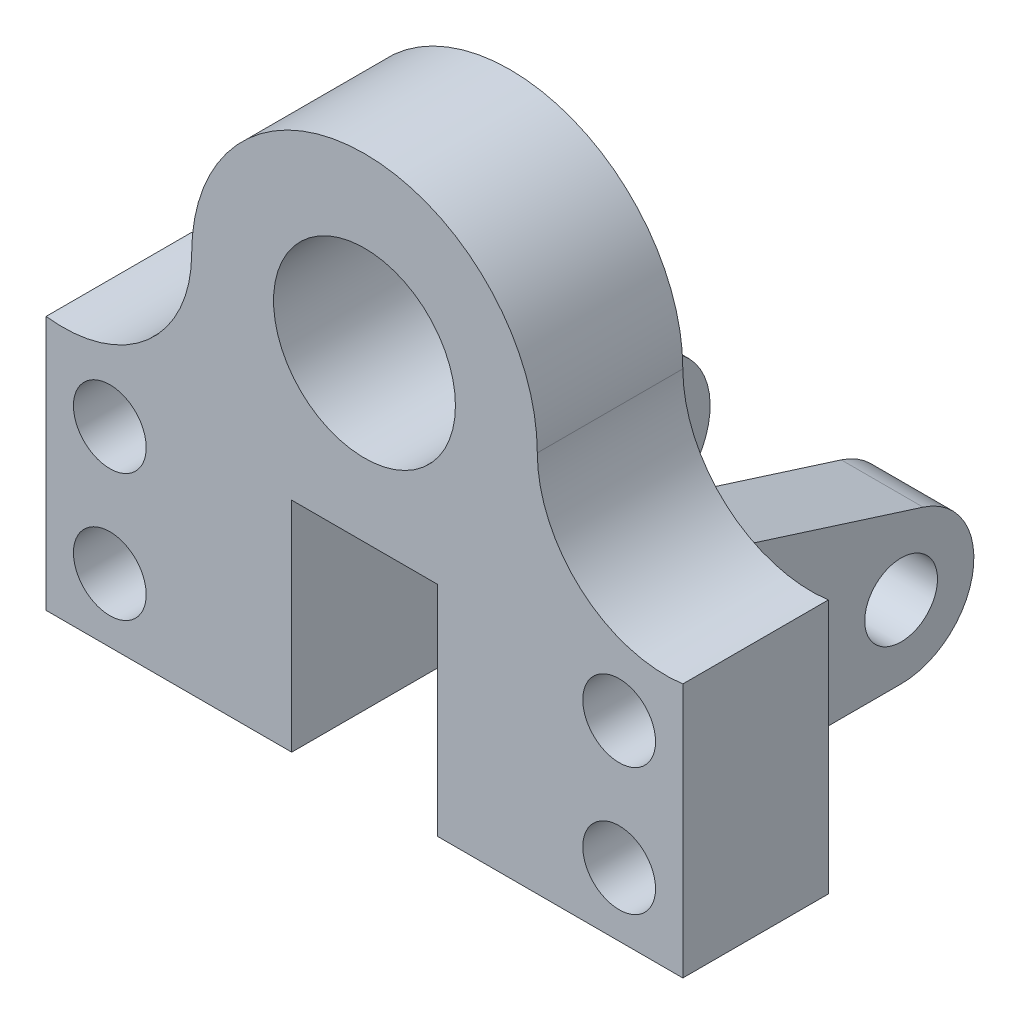
ISO-10303-21;
HEADER;
FILE_DESCRIPTION(('STEP AP214'),'2;1');
FILE_NAME('part.step','',(''),(''),'','','');
FILE_SCHEMA(('AUTOMOTIVE_DESIGN { 1 0 10303 214 1 1 1 1 }'));
ENDSEC;
DATA;
#1=APPLICATION_CONTEXT('core data for automotive mechanical design processes');
#2=APPLICATION_PROTOCOL_DEFINITION('international standard','automotive_design',2000,#1);
#3=PRODUCT_CONTEXT('',#1,'mechanical');
#4=PRODUCT('Part','Part','',(#3));
#5=PRODUCT_RELATED_PRODUCT_CATEGORY('part','',(#4));
#6=PRODUCT_DEFINITION_FORMATION('','',#4);
#7=PRODUCT_DEFINITION_CONTEXT('part definition',#1,'design');
#8=PRODUCT_DEFINITION('design','',#6,#7);
#9=PRODUCT_DEFINITION_SHAPE('','',#8);
#10=(LENGTH_UNIT() NAMED_UNIT(*) SI_UNIT(.MILLI.,.METRE.));
#11=(NAMED_UNIT(*) PLANE_ANGLE_UNIT() SI_UNIT($,.RADIAN.));
#12=(NAMED_UNIT(*) SI_UNIT($,.STERADIAN.) SOLID_ANGLE_UNIT());
#13=UNCERTAINTY_MEASURE_WITH_UNIT(LENGTH_MEASURE(1.E-05),#10,'distance_accuracy_value','');
#14=(GEOMETRIC_REPRESENTATION_CONTEXT(3) GLOBAL_UNCERTAINTY_ASSIGNED_CONTEXT((#13)) GLOBAL_UNIT_ASSIGNED_CONTEXT((#10,
#11,#12)) REPRESENTATION_CONTEXT('',''));
#15=CARTESIAN_POINT('',(0.,0.,0.));
#16=DIRECTION('',(0.,0.,1.));
#17=DIRECTION('',(1.,0.,0.));
#18=AXIS2_PLACEMENT_3D('',#15,#16,#17);
#19=CARTESIAN_POINT('',(-66.25,36.,-16.));
#20=DIRECTION('',(0.,0.,-1.));
#21=DIRECTION('',(-1.,0.,0.));
#22=AXIS2_PLACEMENT_3D('',#19,#20,#21);
#23=PLANE('',#22);
#24=DIRECTION('',(0.,-1.,0.));
#25=VECTOR('',#24,1.);
#26=CARTESIAN_POINT('',(-38.,0.,-16.));
#27=LINE('',#26,#25);
#28=CARTESIAN_POINT('',(-38.,0.,-16.));
#29=VERTEX_POINT('',#28);
#30=CARTESIAN_POINT('',(-38.,-48.,-16.));
#31=VERTEX_POINT('',#30);
#32=EDGE_CURVE('E164',#29,#31,#27,.T.);
#33=ORIENTED_EDGE('',*,*,#32,.T.);
#34=DIRECTION('',(1.,0.,0.));
#35=VECTOR('',#34,1.);
#36=CARTESIAN_POINT('',(-16.,-48.,-16.));
#37=LINE('',#36,#35);
#38=CARTESIAN_POINT('',(-70.,-48.,-16.));
#39=VERTEX_POINT('',#38);
#40=EDGE_CURVE('E283',#39,#31,#37,.T.);
#41=ORIENTED_EDGE('',*,*,#40,.F.);
#42=DIRECTION('',(0.,-1.,0.));
#43=VECTOR('',#42,1.);
#44=CARTESIAN_POINT('',(-70.,-48.,-16.));
#45=LINE('',#44,#43);
#46=CARTESIAN_POINT('',(-70.,8.,-16.));
#47=VERTEX_POINT('',#46);
#48=EDGE_CURVE('E285',#47,#39,#45,.T.);
#49=ORIENTED_EDGE('',*,*,#48,.F.);
#50=CARTESIAN_POINT('',(-66.25,36.,-16.));
#51=DIRECTION('',(0.,0.,-1.));
#52=DIRECTION('',(-1.,0.,0.));
#53=AXIS2_PLACEMENT_3D('',#50,#51,#52);
#54=CIRCLE('',#53,28.25);
#55=CARTESIAN_POINT('',(-38.,36.,-16.));
#56=VERTEX_POINT('',#55);
#57=EDGE_CURVE('E255',#56,#47,#54,.T.);
#58=ORIENTED_EDGE('',*,*,#57,.F.);
#59=CARTESIAN_POINT('',(0.,36.,-16.));
#60=DIRECTION('',(0.,0.,1.));
#61=DIRECTION('',(1.,0.,0.));
#62=AXIS2_PLACEMENT_3D('',#59,#60,#61);
#63=CIRCLE('',#62,38.);
#64=CARTESIAN_POINT('',(38.,36.,-16.));
#65=VERTEX_POINT('',#64);
#66=EDGE_CURVE('E261',#65,#56,#63,.T.);
#67=ORIENTED_EDGE('',*,*,#66,.F.);
#68=CARTESIAN_POINT('',(66.25,36.,-16.));
#69=DIRECTION('',(0.,0.,-1.));
#70=DIRECTION('',(1.,0.,0.));
#71=AXIS2_PLACEMENT_3D('',#68,#69,#70);
#72=CIRCLE('',#71,28.25);
#73=CARTESIAN_POINT('',(70.,8.,-16.));
#74=VERTEX_POINT('',#73);
#75=EDGE_CURVE('E296',#74,#65,#72,.T.);
#76=ORIENTED_EDGE('',*,*,#75,.F.);
#77=DIRECTION('',(0.,1.,0.));
#78=VECTOR('',#77,1.);
#79=CARTESIAN_POINT('',(70.,-48.,-16.));
#80=LINE('',#79,#78);
#81=CARTESIAN_POINT('',(70.,-48.,-16.));
#82=VERTEX_POINT('',#81);
#83=EDGE_CURVE('E300',#82,#74,#80,.T.);
#84=ORIENTED_EDGE('',*,*,#83,.F.);
#85=DIRECTION('',(1.,0.,0.));
#86=VECTOR('',#85,1.);
#87=CARTESIAN_POINT('',(16.,-48.,-16.));
#88=LINE('',#87,#86);
#89=CARTESIAN_POINT('',(38.,-48.,-16.));
#90=VERTEX_POINT('',#89);
#91=EDGE_CURVE('E291',#90,#82,#88,.T.);
#92=ORIENTED_EDGE('',*,*,#91,.F.);
#93=DIRECTION('',(0.,-1.,0.));
#94=VECTOR('',#93,1.);
#95=CARTESIAN_POINT('',(38.,0.,-16.));
#96=LINE('',#95,#94);
#97=CARTESIAN_POINT('',(38.,0.,-16.));
#98=VERTEX_POINT('',#97);
#99=EDGE_CURVE('E203',#98,#90,#96,.T.);
#100=ORIENTED_EDGE('',*,*,#99,.F.);
#101=DIRECTION('',(-1.,0.,0.));
#102=VECTOR('',#101,1.);
#103=CARTESIAN_POINT('',(38.,0.,-16.));
#104=LINE('',#103,#102);
#105=CARTESIAN_POINT('',(20.,0.,-16.));
#106=VERTEX_POINT('',#105);
#107=EDGE_CURVE('E211',#98,#106,#104,.T.);
#108=ORIENTED_EDGE('',*,*,#107,.T.);
#109=DIRECTION('',(0.,-1.,0.));
#110=VECTOR('',#109,1.);
#111=CARTESIAN_POINT('',(20.,0.,-16.));
#112=LINE('',#111,#110);
#113=CARTESIAN_POINT('',(20.,-48.,-16.));
#114=VERTEX_POINT('',#113);
#115=EDGE_CURVE('E65',#106,#114,#112,.T.);
#116=ORIENTED_EDGE('',*,*,#115,.T.);
#117=CARTESIAN_POINT('',(16.,-48.,-16.));
#118=VERTEX_POINT('',#117);
#119=EDGE_CURVE('E294',#118,#114,#88,.T.);
#120=ORIENTED_EDGE('',*,*,#119,.F.);
#121=DIRECTION('',(0.,-1.,0.));
#122=VECTOR('',#121,1.);
#123=CARTESIAN_POINT('',(16.,0.,-16.));
#124=LINE('',#123,#122);
#125=CARTESIAN_POINT('',(16.,0.,-16.));
#126=VERTEX_POINT('',#125);
#127=EDGE_CURVE('E292',#126,#118,#124,.T.);
#128=ORIENTED_EDGE('',*,*,#127,.F.);
#129=DIRECTION('',(1.,0.,0.));
#130=VECTOR('',#129,1.);
#131=CARTESIAN_POINT('',(-16.,0.,-16.));
#132=LINE('',#131,#130);
#133=CARTESIAN_POINT('',(-16.,0.,-16.));
#134=VERTEX_POINT('',#133);
#135=EDGE_CURVE('E287',#134,#126,#132,.T.);
#136=ORIENTED_EDGE('',*,*,#135,.F.);
#137=DIRECTION('',(0.,1.,0.));
#138=VECTOR('',#137,1.);
#139=CARTESIAN_POINT('',(-16.,0.,-16.));
#140=LINE('',#139,#138);
#141=CARTESIAN_POINT('',(-16.,-48.,-16.));
#142=VERTEX_POINT('',#141);
#143=EDGE_CURVE('E290',#142,#134,#140,.T.);
#144=ORIENTED_EDGE('',*,*,#143,.F.);
#145=CARTESIAN_POINT('',(-20.,-48.,-16.));
#146=VERTEX_POINT('',#145);
#147=EDGE_CURVE('E281',#146,#142,#37,.T.);
#148=ORIENTED_EDGE('',*,*,#147,.F.);
#149=DIRECTION('',(0.,-1.,0.));
#150=VECTOR('',#149,1.);
#151=CARTESIAN_POINT('',(-20.,0.,-16.));
#152=LINE('',#151,#150);
#153=CARTESIAN_POINT('',(-20.,0.,-16.));
#154=VERTEX_POINT('',#153);
#155=EDGE_CURVE('E186',#154,#146,#152,.T.);
#156=ORIENTED_EDGE('',*,*,#155,.F.);
#157=DIRECTION('',(1.,0.,0.));
#158=VECTOR('',#157,1.);
#159=CARTESIAN_POINT('',(-38.,0.,-16.));
#160=LINE('',#159,#158);
#161=EDGE_CURVE('E182',#29,#154,#160,.T.);
#162=ORIENTED_EDGE('',*,*,#161,.F.);
#163=EDGE_LOOP('',(#33,#41,#49,#58,#67,#76,#84,#92,#100,#108,#116,#120,#128,#136,#144,#148,#156,#162));
#164=FACE_BOUND('',#163,.T.);
#165=CARTESIAN_POINT('',(-56.,-34.,-16.));
#166=DIRECTION('',(0.,0.,1.));
#167=DIRECTION('',(-1.,0.,0.));
#168=AXIS2_PLACEMENT_3D('',#165,#166,#167);
#169=CIRCLE('',#168,8.00000000000001);
#170=CARTESIAN_POINT('',(-64.,-34.,-16.));
#171=VERTEX_POINT('',#170);
#172=EDGE_CURVE('E228',#171,#171,#169,.T.);
#173=ORIENTED_EDGE('',*,*,#172,.T.);
#174=EDGE_LOOP('',(#173));
#175=FACE_BOUND('',#174,.T.);
#176=CARTESIAN_POINT('',(56.,-34.,-16.));
#177=DIRECTION('',(0.,0.,1.));
#178=DIRECTION('',(1.,0.,0.));
#179=AXIS2_PLACEMENT_3D('',#176,#177,#178);
#180=CIRCLE('',#179,8.00000000000001);
#181=CARTESIAN_POINT('',(64.,-34.,-16.));
#182=VERTEX_POINT('',#181);
#183=EDGE_CURVE('E245',#182,#182,#180,.T.);
#184=ORIENTED_EDGE('',*,*,#183,.T.);
#185=EDGE_LOOP('',(#184));
#186=FACE_BOUND('',#185,.T.);
#187=CARTESIAN_POINT('',(0.,36.,-16.));
#188=DIRECTION('',(0.,0.,1.));
#189=DIRECTION('',(1.,0.,0.));
#190=AXIS2_PLACEMENT_3D('',#187,#188,#189);
#191=CIRCLE('',#190,20.);
#192=CARTESIAN_POINT('',(20.,36.,-16.));
#193=VERTEX_POINT('',#192);
#194=EDGE_CURVE('E246',#193,#193,#191,.T.);
#195=ORIENTED_EDGE('',*,*,#194,.T.);
#196=EDGE_LOOP('',(#195));
#197=FACE_BOUND('',#196,.T.);
#198=CARTESIAN_POINT('',(56.,-6.,-16.));
#199=DIRECTION('',(0.,0.,1.));
#200=DIRECTION('',(1.,0.,0.));
#201=AXIS2_PLACEMENT_3D('',#198,#199,#200);
#202=CIRCLE('',#201,8.);
#203=CARTESIAN_POINT('',(64.,-6.,-16.));
#204=VERTEX_POINT('',#203);
#205=EDGE_CURVE('E237',#204,#204,#202,.T.);
#206=ORIENTED_EDGE('',*,*,#205,.T.);
#207=EDGE_LOOP('',(#206));
#208=FACE_BOUND('',#207,.T.);
#209=CARTESIAN_POINT('',(-56.,-6.00000000000003,-16.));
#210=DIRECTION('',(0.,0.,1.));
#211=DIRECTION('',(-1.,0.,0.));
#212=AXIS2_PLACEMENT_3D('',#209,#210,#211);
#213=CIRCLE('',#212,8.);
#214=CARTESIAN_POINT('',(-64.,-6.00000000000003,-16.));
#215=VERTEX_POINT('',#214);
#216=EDGE_CURVE('E227',#215,#215,#213,.T.);
#217=ORIENTED_EDGE('',*,*,#216,.T.);
#218=EDGE_LOOP('',(#217));
#219=FACE_BOUND('',#218,.T.);
#220=ADVANCED_FACE('F39',(#164,#175,#186,#197,#208,#219),#23,.T.);
#221=CARTESIAN_POINT('',(-66.25,36.,16.));
#222=DIRECTION('',(0.,0.,-1.));
#223=DIRECTION('',(-1.,0.,0.));
#224=AXIS2_PLACEMENT_3D('',#221,#222,#223);
#225=PLANE('',#224);
#226=CARTESIAN_POINT('',(-66.25,36.,16.));
#227=DIRECTION('',(0.,0.,-1.));
#228=DIRECTION('',(-1.,0.,0.));
#229=AXIS2_PLACEMENT_3D('',#226,#227,#228);
#230=CIRCLE('',#229,28.25);
#231=CARTESIAN_POINT('',(-38.,36.,16.));
#232=VERTEX_POINT('',#231);
#233=CARTESIAN_POINT('',(-70.,8.,16.));
#234=VERTEX_POINT('',#233);
#235=EDGE_CURVE('E260',#232,#234,#230,.T.);
#236=ORIENTED_EDGE('',*,*,#235,.T.);
#237=DIRECTION('',(0.,-1.,0.));
#238=VECTOR('',#237,1.);
#239=CARTESIAN_POINT('',(-70.,-48.,16.));
#240=LINE('',#239,#238);
#241=CARTESIAN_POINT('',(-70.,-48.,16.));
#242=VERTEX_POINT('',#241);
#243=EDGE_CURVE('E257',#234,#242,#240,.T.);
#244=ORIENTED_EDGE('',*,*,#243,.T.);
#245=DIRECTION('',(1.,0.,0.));
#246=VECTOR('',#245,1.);
#247=CARTESIAN_POINT('',(-16.,-48.,16.));
#248=LINE('',#247,#246);
#249=CARTESIAN_POINT('',(-16.,-48.,16.));
#250=VERTEX_POINT('',#249);
#251=EDGE_CURVE('E263',#242,#250,#248,.T.);
#252=ORIENTED_EDGE('',*,*,#251,.T.);
#253=DIRECTION('',(0.,1.,0.));
#254=VECTOR('',#253,1.);
#255=CARTESIAN_POINT('',(-16.,0.,16.));
#256=LINE('',#255,#254);
#257=CARTESIAN_POINT('',(-16.,0.,16.));
#258=VERTEX_POINT('',#257);
#259=EDGE_CURVE('E264',#250,#258,#256,.T.);
#260=ORIENTED_EDGE('',*,*,#259,.T.);
#261=DIRECTION('',(1.,0.,0.));
#262=VECTOR('',#261,1.);
#263=CARTESIAN_POINT('',(-16.,0.,16.));
#264=LINE('',#263,#262);
#265=CARTESIAN_POINT('',(16.,0.,16.));
#266=VERTEX_POINT('',#265);
#267=EDGE_CURVE('E270',#258,#266,#264,.T.);
#268=ORIENTED_EDGE('',*,*,#267,.T.);
#269=DIRECTION('',(0.,-1.,0.));
#270=VECTOR('',#269,1.);
#271=CARTESIAN_POINT('',(16.,0.,16.));
#272=LINE('',#271,#270);
#273=CARTESIAN_POINT('',(16.,-48.,16.));
#274=VERTEX_POINT('',#273);
#275=EDGE_CURVE('E267',#266,#274,#272,.T.);
#276=ORIENTED_EDGE('',*,*,#275,.T.);
#277=DIRECTION('',(1.,0.,0.));
#278=VECTOR('',#277,1.);
#279=CARTESIAN_POINT('',(16.,-48.,16.));
#280=LINE('',#279,#278);
#281=CARTESIAN_POINT('',(70.,-48.,16.));
#282=VERTEX_POINT('',#281);
#283=EDGE_CURVE('E271',#274,#282,#280,.T.);
#284=ORIENTED_EDGE('',*,*,#283,.T.);
#285=DIRECTION('',(0.,1.,0.));
#286=VECTOR('',#285,1.);
#287=CARTESIAN_POINT('',(70.,-48.,16.));
#288=LINE('',#287,#286);
#289=CARTESIAN_POINT('',(70.,8.,16.));
#290=VERTEX_POINT('',#289);
#291=EDGE_CURVE('E272',#282,#290,#288,.T.);
#292=ORIENTED_EDGE('',*,*,#291,.T.);
#293=CARTESIAN_POINT('',(66.25,36.,16.));
#294=DIRECTION('',(0.,0.,-1.));
#295=DIRECTION('',(1.,0.,0.));
#296=AXIS2_PLACEMENT_3D('',#293,#294,#295);
#297=CIRCLE('',#296,28.25);
#298=CARTESIAN_POINT('',(38.,36.,16.));
#299=VERTEX_POINT('',#298);
#300=EDGE_CURVE('E274',#290,#299,#297,.T.);
#301=ORIENTED_EDGE('',*,*,#300,.T.);
#302=CARTESIAN_POINT('',(0.,36.,16.));
#303=DIRECTION('',(0.,0.,1.));
#304=DIRECTION('',(1.,0.,0.));
#305=AXIS2_PLACEMENT_3D('',#302,#303,#304);
#306=CIRCLE('',#305,38.);
#307=EDGE_CURVE('E280',#299,#232,#306,.T.);
#308=ORIENTED_EDGE('',*,*,#307,.T.);
#309=EDGE_LOOP('',(#236,#244,#252,#260,#268,#276,#284,#292,#301,#308));
#310=FACE_BOUND('',#309,.T.);
#311=CARTESIAN_POINT('',(0.,36.,16.));
#312=DIRECTION('',(0.,0.,1.));
#313=DIRECTION('',(1.,0.,0.));
#314=AXIS2_PLACEMENT_3D('',#311,#312,#313);
#315=CIRCLE('',#314,20.);
#316=CARTESIAN_POINT('',(20.,36.,16.));
#317=VERTEX_POINT('',#316);
#318=EDGE_CURVE('E253',#317,#317,#315,.T.);
#319=ORIENTED_EDGE('',*,*,#318,.F.);
#320=EDGE_LOOP('',(#319));
#321=FACE_BOUND('',#320,.T.);
#322=CARTESIAN_POINT('',(56.,-34.,16.));
#323=DIRECTION('',(0.,0.,1.));
#324=DIRECTION('',(1.,0.,0.));
#325=AXIS2_PLACEMENT_3D('',#322,#323,#324);
#326=CIRCLE('',#325,8.00000000000001);
#327=CARTESIAN_POINT('',(64.,-34.,16.));
#328=VERTEX_POINT('',#327);
#329=EDGE_CURVE('E243',#328,#328,#326,.T.);
#330=ORIENTED_EDGE('',*,*,#329,.F.);
#331=EDGE_LOOP('',(#330));
#332=FACE_BOUND('',#331,.T.);
#333=CARTESIAN_POINT('',(56.,-6.,16.));
#334=DIRECTION('',(0.,0.,1.));
#335=DIRECTION('',(1.,0.,0.));
#336=AXIS2_PLACEMENT_3D('',#333,#334,#335);
#337=CIRCLE('',#336,8.);
#338=CARTESIAN_POINT('',(64.,-6.,16.));
#339=VERTEX_POINT('',#338);
#340=EDGE_CURVE('E239',#339,#339,#337,.T.);
#341=ORIENTED_EDGE('',*,*,#340,.F.);
#342=EDGE_LOOP('',(#341));
#343=FACE_BOUND('',#342,.T.);
#344=CARTESIAN_POINT('',(-56.,-34.,16.));
#345=DIRECTION('',(0.,0.,1.));
#346=DIRECTION('',(-1.,0.,0.));
#347=AXIS2_PLACEMENT_3D('',#344,#345,#346);
#348=CIRCLE('',#347,8.00000000000001);
#349=CARTESIAN_POINT('',(-64.,-34.,16.));
#350=VERTEX_POINT('',#349);
#351=EDGE_CURVE('E231',#350,#350,#348,.T.);
#352=ORIENTED_EDGE('',*,*,#351,.F.);
#353=EDGE_LOOP('',(#352));
#354=FACE_BOUND('',#353,.T.);
#355=CARTESIAN_POINT('',(-56.,-6.00000000000003,16.));
#356=DIRECTION('',(0.,0.,1.));
#357=DIRECTION('',(-1.,0.,0.));
#358=AXIS2_PLACEMENT_3D('',#355,#356,#357);
#359=CIRCLE('',#358,8.);
#360=CARTESIAN_POINT('',(-64.,-6.00000000000003,16.));
#361=VERTEX_POINT('',#360);
#362=EDGE_CURVE('E230',#361,#361,#359,.T.);
#363=ORIENTED_EDGE('',*,*,#362,.F.);
#364=EDGE_LOOP('',(#363));
#365=FACE_BOUND('',#364,.T.);
#366=ADVANCED_FACE('F389',(#310,#321,#332,#343,#354,#365),#225,.F.);
#367=CARTESIAN_POINT('',(-66.25,36.,16.));
#368=DIRECTION('',(0.,0.,-1.));
#369=DIRECTION('',(-1.,0.,0.));
#370=AXIS2_PLACEMENT_3D('',#367,#368,#369);
#371=CYLINDRICAL_SURFACE('',#370,28.25);
#372=ORIENTED_EDGE('',*,*,#57,.T.);
#373=DIRECTION('',(0.,0.,-1.));
#374=VECTOR('',#373,1.);
#375=CARTESIAN_POINT('',(-70.,8.,16.));
#376=LINE('',#375,#374);
#377=EDGE_CURVE('E11',#234,#47,#376,.T.);
#378=ORIENTED_EDGE('',*,*,#377,.F.);
#379=ORIENTED_EDGE('',*,*,#235,.F.);
#380=DIRECTION('',(0.,0.,-1.));
#381=VECTOR('',#380,1.);
#382=CARTESIAN_POINT('',(-38.,36.,16.));
#383=LINE('',#382,#381);
#384=EDGE_CURVE('E276',#232,#56,#383,.T.);
#385=ORIENTED_EDGE('',*,*,#384,.T.);
#386=EDGE_LOOP('',(#372,#378,#379,#385));
#387=FACE_BOUND('',#386,.T.);
#388=ADVANCED_FACE('F41',(#387),#371,.F.);
#389=CARTESIAN_POINT('',(-70.,-48.,16.));
#390=DIRECTION('',(1.,0.,0.));
#391=DIRECTION('',(0.,0.,-1.));
#392=AXIS2_PLACEMENT_3D('',#389,#390,#391);
#393=PLANE('',#392);
#394=ORIENTED_EDGE('',*,*,#48,.T.);
#395=DIRECTION('',(0.,0.,-1.));
#396=VECTOR('',#395,1.);
#397=CARTESIAN_POINT('',(-70.,-48.,16.));
#398=LINE('',#397,#396);
#399=EDGE_CURVE('E50',#242,#39,#398,.T.);
#400=ORIENTED_EDGE('',*,*,#399,.F.);
#401=ORIENTED_EDGE('',*,*,#243,.F.);
#402=ORIENTED_EDGE('',*,*,#377,.T.);
#403=EDGE_LOOP('',(#394,#400,#401,#402));
#404=FACE_BOUND('',#403,.T.);
#405=ADVANCED_FACE('F334',(#404),#393,.F.);
#406=CARTESIAN_POINT('',(-16.,-48.,16.));
#407=DIRECTION('',(0.,1.,0.));
#408=DIRECTION('',(0.,0.,1.));
#409=AXIS2_PLACEMENT_3D('',#406,#407,#408);
#410=PLANE('',#409);
#411=ORIENTED_EDGE('',*,*,#40,.T.);
#412=DIRECTION('',(0.,0.,-1.));
#413=VECTOR('',#412,1.);
#414=CARTESIAN_POINT('',(-38.,-48.,-16.));
#415=LINE('',#414,#413);
#416=CARTESIAN_POINT('',(-38.,-48.,-64.));
#417=VERTEX_POINT('',#416);
#418=EDGE_CURVE('E175',#31,#417,#415,.T.);
#419=ORIENTED_EDGE('',*,*,#418,.T.);
#420=DIRECTION('',(1.,0.,0.));
#421=VECTOR('',#420,1.);
#422=CARTESIAN_POINT('',(-38.,-48.,-64.));
#423=LINE('',#422,#421);
#424=CARTESIAN_POINT('',(-20.,-48.,-64.));
#425=VERTEX_POINT('',#424);
#426=EDGE_CURVE('E194',#417,#425,#423,.T.);
#427=ORIENTED_EDGE('',*,*,#426,.T.);
#428=DIRECTION('',(0.,0.,-1.));
#429=VECTOR('',#428,1.);
#430=CARTESIAN_POINT('',(-20.,-48.,-16.));
#431=LINE('',#430,#429);
#432=EDGE_CURVE('E53',#146,#425,#431,.T.);
#433=ORIENTED_EDGE('',*,*,#432,.F.);
#434=ORIENTED_EDGE('',*,*,#147,.T.);
#435=DIRECTION('',(0.,0.,-1.));
#436=VECTOR('',#435,1.);
#437=CARTESIAN_POINT('',(-16.,-48.,16.));
#438=LINE('',#437,#436);
#439=EDGE_CURVE('E325',#250,#142,#438,.T.);
#440=ORIENTED_EDGE('',*,*,#439,.F.);
#441=ORIENTED_EDGE('',*,*,#251,.F.);
#442=ORIENTED_EDGE('',*,*,#399,.T.);
#443=EDGE_LOOP('',(#411,#419,#427,#433,#434,#440,#441,#442));
#444=FACE_BOUND('',#443,.T.);
#445=ADVANCED_FACE('F330',(#444),#410,.F.);
#446=CARTESIAN_POINT('',(-16.,0.,16.));
#447=DIRECTION('',(-1.,0.,0.));
#448=DIRECTION('',(0.,-1.,0.));
#449=AXIS2_PLACEMENT_3D('',#446,#447,#448);
#450=PLANE('',#449);
#451=ORIENTED_EDGE('',*,*,#143,.T.);
#452=DIRECTION('',(0.,0.,-1.));
#453=VECTOR('',#452,1.);
#454=CARTESIAN_POINT('',(-16.,0.,16.));
#455=LINE('',#454,#453);
#456=EDGE_CURVE('E317',#258,#134,#455,.T.);
#457=ORIENTED_EDGE('',*,*,#456,.F.);
#458=ORIENTED_EDGE('',*,*,#259,.F.);
#459=ORIENTED_EDGE('',*,*,#439,.T.);
#460=EDGE_LOOP('',(#451,#457,#458,#459));
#461=FACE_BOUND('',#460,.T.);
#462=ADVANCED_FACE('F387',(#461),#450,.F.);
#463=CARTESIAN_POINT('',(-16.,0.,16.));
#464=DIRECTION('',(0.,1.,0.));
#465=DIRECTION('',(0.,0.,1.));
#466=AXIS2_PLACEMENT_3D('',#463,#464,#465);
#467=PLANE('',#466);
#468=ORIENTED_EDGE('',*,*,#135,.T.);
#469=DIRECTION('',(0.,0.,-1.));
#470=VECTOR('',#469,1.);
#471=CARTESIAN_POINT('',(16.,0.,16.));
#472=LINE('',#471,#470);
#473=EDGE_CURVE('E316',#266,#126,#472,.T.);
#474=ORIENTED_EDGE('',*,*,#473,.F.);
#475=ORIENTED_EDGE('',*,*,#267,.F.);
#476=ORIENTED_EDGE('',*,*,#456,.T.);
#477=EDGE_LOOP('',(#468,#474,#475,#476));
#478=FACE_BOUND('',#477,.T.);
#479=ADVANCED_FACE('F385',(#478),#467,.F.);
#480=CARTESIAN_POINT('',(16.,0.,16.));
#481=DIRECTION('',(1.,0.,0.));
#482=DIRECTION('',(0.,1.,0.));
#483=AXIS2_PLACEMENT_3D('',#480,#481,#482);
#484=PLANE('',#483);
#485=ORIENTED_EDGE('',*,*,#127,.T.);
#486=DIRECTION('',(0.,0.,-1.));
#487=VECTOR('',#486,1.);
#488=CARTESIAN_POINT('',(16.,-48.,16.));
#489=LINE('',#488,#487);
#490=EDGE_CURVE('E311',#274,#118,#489,.T.);
#491=ORIENTED_EDGE('',*,*,#490,.F.);
#492=ORIENTED_EDGE('',*,*,#275,.F.);
#493=ORIENTED_EDGE('',*,*,#473,.T.);
#494=EDGE_LOOP('',(#485,#491,#492,#493));
#495=FACE_BOUND('',#494,.T.);
#496=ADVANCED_FACE('F380',(#495),#484,.F.);
#497=CARTESIAN_POINT('',(16.,-48.,16.));
#498=DIRECTION('',(0.,1.,0.));
#499=DIRECTION('',(0.,0.,1.));
#500=AXIS2_PLACEMENT_3D('',#497,#498,#499);
#501=PLANE('',#500);
#502=ORIENTED_EDGE('',*,*,#119,.T.);
#503=DIRECTION('',(0.,0.,-1.));
#504=VECTOR('',#503,1.);
#505=CARTESIAN_POINT('',(20.,-48.,-16.));
#506=LINE('',#505,#504);
#507=CARTESIAN_POINT('',(20.,-48.,-64.));
#508=VERTEX_POINT('',#507);
#509=EDGE_CURVE('E213',#114,#508,#506,.T.);
#510=ORIENTED_EDGE('',*,*,#509,.T.);
#511=DIRECTION('',(-1.,0.,0.));
#512=VECTOR('',#511,1.);
#513=CARTESIAN_POINT('',(38.,-48.,-64.));
#514=LINE('',#513,#512);
#515=CARTESIAN_POINT('',(38.,-48.,-64.));
#516=VERTEX_POINT('',#515);
#517=EDGE_CURVE('E224',#516,#508,#514,.T.);
#518=ORIENTED_EDGE('',*,*,#517,.F.);
#519=DIRECTION('',(0.,0.,-1.));
#520=VECTOR('',#519,1.);
#521=CARTESIAN_POINT('',(38.,-48.,-16.));
#522=LINE('',#521,#520);
#523=EDGE_CURVE('E204',#90,#516,#522,.T.);
#524=ORIENTED_EDGE('',*,*,#523,.F.);
#525=ORIENTED_EDGE('',*,*,#91,.T.);
#526=DIRECTION('',(0.,0.,-1.));
#527=VECTOR('',#526,1.);
#528=CARTESIAN_POINT('',(70.,-48.,16.));
#529=LINE('',#528,#527);
#530=EDGE_CURVE('E309',#282,#82,#529,.T.);
#531=ORIENTED_EDGE('',*,*,#530,.F.);
#532=ORIENTED_EDGE('',*,*,#283,.F.);
#533=ORIENTED_EDGE('',*,*,#490,.T.);
#534=EDGE_LOOP('',(#502,#510,#518,#524,#525,#531,#532,#533));
#535=FACE_BOUND('',#534,.T.);
#536=ADVANCED_FACE('F351',(#535),#501,.F.);
#537=CARTESIAN_POINT('',(70.,-48.,16.));
#538=DIRECTION('',(-1.,0.,0.));
#539=DIRECTION('',(0.,0.,1.));
#540=AXIS2_PLACEMENT_3D('',#537,#538,#539);
#541=PLANE('',#540);
#542=ORIENTED_EDGE('',*,*,#83,.T.);
#543=DIRECTION('',(0.,0.,-1.));
#544=VECTOR('',#543,1.);
#545=CARTESIAN_POINT('',(70.,8.,16.));
#546=LINE('',#545,#544);
#547=EDGE_CURVE('E307',#290,#74,#546,.T.);
#548=ORIENTED_EDGE('',*,*,#547,.F.);
#549=ORIENTED_EDGE('',*,*,#291,.F.);
#550=ORIENTED_EDGE('',*,*,#530,.T.);
#551=EDGE_LOOP('',(#542,#548,#549,#550));
#552=FACE_BOUND('',#551,.T.);
#553=ADVANCED_FACE('F348',(#552),#541,.F.);
#554=CARTESIAN_POINT('',(66.25,36.,16.));
#555=DIRECTION('',(0.,0.,-1.));
#556=DIRECTION('',(-1.,0.,0.));
#557=AXIS2_PLACEMENT_3D('',#554,#555,#556);
#558=CYLINDRICAL_SURFACE('',#557,28.25);
#559=ORIENTED_EDGE('',*,*,#75,.T.);
#560=DIRECTION('',(0.,0.,-1.));
#561=VECTOR('',#560,1.);
#562=CARTESIAN_POINT('',(38.,36.,16.));
#563=LINE('',#562,#561);
#564=EDGE_CURVE('E302',#299,#65,#563,.T.);
#565=ORIENTED_EDGE('',*,*,#564,.F.);
#566=ORIENTED_EDGE('',*,*,#300,.F.);
#567=ORIENTED_EDGE('',*,*,#547,.T.);
#568=EDGE_LOOP('',(#559,#565,#566,#567));
#569=FACE_BOUND('',#568,.T.);
#570=ADVANCED_FACE('F344',(#569),#558,.F.);
#571=CARTESIAN_POINT('',(0.,36.,16.));
#572=DIRECTION('',(0.,0.,-1.));
#573=DIRECTION('',(-1.,0.,0.));
#574=AXIS2_PLACEMENT_3D('',#571,#572,#573);
#575=CYLINDRICAL_SURFACE('',#574,38.);
#576=ORIENTED_EDGE('',*,*,#66,.T.);
#577=ORIENTED_EDGE('',*,*,#384,.F.);
#578=ORIENTED_EDGE('',*,*,#307,.F.);
#579=ORIENTED_EDGE('',*,*,#564,.T.);
#580=EDGE_LOOP('',(#576,#577,#578,#579));
#581=FACE_BOUND('',#580,.T.);
#582=ADVANCED_FACE('F336',(#581),#575,.T.);
#583=CARTESIAN_POINT('',(0.,36.,16.));
#584=DIRECTION('',(0.,0.,-1.));
#585=DIRECTION('',(-1.,0.,0.));
#586=AXIS2_PLACEMENT_3D('',#583,#584,#585);
#587=CYLINDRICAL_SURFACE('',#586,20.);
#588=ORIENTED_EDGE('',*,*,#318,.T.);
#589=EDGE_LOOP('',(#588));
#590=FACE_BOUND('',#589,.T.);
#591=ORIENTED_EDGE('',*,*,#194,.F.);
#592=EDGE_LOOP('',(#591));
#593=FACE_BOUND('',#592,.T.);
#594=ADVANCED_FACE('F420',(#590,#593),#587,.F.);
#595=CARTESIAN_POINT('',(56.,-34.,16.));
#596=DIRECTION('',(0.,0.,-1.));
#597=DIRECTION('',(-1.,0.,0.));
#598=AXIS2_PLACEMENT_3D('',#595,#596,#597);
#599=CYLINDRICAL_SURFACE('',#598,8.00000000000001);
#600=ORIENTED_EDGE('',*,*,#329,.T.);
#601=EDGE_LOOP('',(#600));
#602=FACE_BOUND('',#601,.T.);
#603=ORIENTED_EDGE('',*,*,#183,.F.);
#604=EDGE_LOOP('',(#603));
#605=FACE_BOUND('',#604,.T.);
#606=ADVANCED_FACE('F496',(#602,#605),#599,.F.);
#607=CARTESIAN_POINT('',(56.,-6.,16.));
#608=DIRECTION('',(0.,0.,-1.));
#609=DIRECTION('',(-1.,0.,0.));
#610=AXIS2_PLACEMENT_3D('',#607,#608,#609);
#611=CYLINDRICAL_SURFACE('',#610,8.);
#612=ORIENTED_EDGE('',*,*,#340,.T.);
#613=EDGE_LOOP('',(#612));
#614=FACE_BOUND('',#613,.T.);
#615=ORIENTED_EDGE('',*,*,#205,.F.);
#616=EDGE_LOOP('',(#615));
#617=FACE_BOUND('',#616,.T.);
#618=ADVANCED_FACE('F510',(#614,#617),#611,.F.);
#619=CARTESIAN_POINT('',(-56.,-34.,16.));
#620=DIRECTION('',(0.,0.,-1.));
#621=DIRECTION('',(-1.,0.,0.));
#622=AXIS2_PLACEMENT_3D('',#619,#620,#621);
#623=CYLINDRICAL_SURFACE('',#622,8.00000000000001);
#624=ORIENTED_EDGE('',*,*,#351,.T.);
#625=EDGE_LOOP('',(#624));
#626=FACE_BOUND('',#625,.T.);
#627=ORIENTED_EDGE('',*,*,#172,.F.);
#628=EDGE_LOOP('',(#627));
#629=FACE_BOUND('',#628,.T.);
#630=ADVANCED_FACE('F403',(#626,#629),#623,.F.);
#631=CARTESIAN_POINT('',(-56.,-6.00000000000003,16.));
#632=DIRECTION('',(0.,0.,-1.));
#633=DIRECTION('',(-1.,0.,0.));
#634=AXIS2_PLACEMENT_3D('',#631,#632,#633);
#635=CYLINDRICAL_SURFACE('',#634,8.);
#636=ORIENTED_EDGE('',*,*,#362,.T.);
#637=EDGE_LOOP('',(#636));
#638=FACE_BOUND('',#637,.T.);
#639=ORIENTED_EDGE('',*,*,#216,.F.);
#640=EDGE_LOOP('',(#639));
#641=FACE_BOUND('',#640,.T.);
#642=ADVANCED_FACE('F405',(#638,#641),#635,.F.);
#643=CARTESIAN_POINT('',(38.,-32.,-64.));
#644=DIRECTION('',(1.,0.,0.));
#645=DIRECTION('',(0.,0.,-1.));
#646=AXIS2_PLACEMENT_3D('',#643,#644,#645);
#647=PLANE('',#646);
#648=ORIENTED_EDGE('',*,*,#99,.T.);
#649=ORIENTED_EDGE('',*,*,#523,.T.);
#650=CARTESIAN_POINT('',(38.,-32.,-64.));
#651=DIRECTION('',(1.,0.,0.));
#652=DIRECTION('',(0.,0.,-1.));
#653=AXIS2_PLACEMENT_3D('',#650,#651,#652);
#654=CIRCLE('',#653,16.);
#655=CARTESIAN_POINT('',(38.,-16.7479324979529,-68.8347116680314));
#656=VERTEX_POINT('',#655);
#657=EDGE_CURVE('E210',#516,#656,#654,.T.);
#658=ORIENTED_EDGE('',*,*,#657,.T.);
#659=DIRECTION('',(0.,0.302169479251963,0.953254218877943));
#660=VECTOR('',#659,1.);
#661=CARTESIAN_POINT('',(38.,0.,-16.));
#662=LINE('',#661,#660);
#663=EDGE_CURVE('E207',#656,#98,#662,.T.);
#664=ORIENTED_EDGE('',*,*,#663,.T.);
#665=EDGE_LOOP('',(#648,#649,#658,#664));
#666=FACE_BOUND('',#665,.T.);
#667=CARTESIAN_POINT('',(38.,-32.,-64.));
#668=DIRECTION('',(1.,0.,0.));
#669=DIRECTION('',(0.,0.,-1.));
#670=AXIS2_PLACEMENT_3D('',#667,#668,#669);
#671=CIRCLE('',#670,8.00000000000001);
#672=CARTESIAN_POINT('',(38.,-32.,-72.));
#673=VERTEX_POINT('',#672);
#674=EDGE_CURVE('E191',#673,#673,#671,.T.);
#675=ORIENTED_EDGE('',*,*,#674,.F.);
#676=EDGE_LOOP('',(#675));
#677=FACE_BOUND('',#676,.T.);
#678=ADVANCED_FACE('F357',(#666,#677),#647,.T.);
#679=CARTESIAN_POINT('',(20.,-32.,-64.));
#680=DIRECTION('',(1.,0.,0.));
#681=DIRECTION('',(0.,0.,-1.));
#682=AXIS2_PLACEMENT_3D('',#679,#680,#681);
#683=PLANE('',#682);
#684=ORIENTED_EDGE('',*,*,#115,.F.);
#685=DIRECTION('',(0.,0.302169479251963,0.953254218877943));
#686=VECTOR('',#685,1.);
#687=CARTESIAN_POINT('',(20.,0.,-16.));
#688=LINE('',#687,#686);
#689=CARTESIAN_POINT('',(20.,-16.7479324979529,-68.8347116680314));
#690=VERTEX_POINT('',#689);
#691=EDGE_CURVE('E202',#690,#106,#688,.T.);
#692=ORIENTED_EDGE('',*,*,#691,.F.);
#693=CARTESIAN_POINT('',(20.,-32.,-64.));
#694=DIRECTION('',(1.,0.,0.));
#695=DIRECTION('',(0.,0.,-1.));
#696=AXIS2_PLACEMENT_3D('',#693,#694,#695);
#697=CIRCLE('',#696,16.);
#698=EDGE_CURVE('E214',#508,#690,#697,.T.);
#699=ORIENTED_EDGE('',*,*,#698,.F.);
#700=ORIENTED_EDGE('',*,*,#509,.F.);
#701=EDGE_LOOP('',(#684,#692,#699,#700));
#702=FACE_BOUND('',#701,.T.);
#703=CARTESIAN_POINT('',(20.,-32.,-64.));
#704=DIRECTION('',(1.,0.,0.));
#705=DIRECTION('',(0.,0.,-1.));
#706=AXIS2_PLACEMENT_3D('',#703,#704,#705);
#707=CIRCLE('',#706,8.00000000000001);
#708=CARTESIAN_POINT('',(20.,-32.,-72.));
#709=VERTEX_POINT('',#708);
#710=EDGE_CURVE('E188',#709,#709,#707,.T.);
#711=ORIENTED_EDGE('',*,*,#710,.T.);
#712=EDGE_LOOP('',(#711));
#713=FACE_BOUND('',#712,.T.);
#714=ADVANCED_FACE('F370',(#702,#713),#683,.F.);
#715=CARTESIAN_POINT('',(38.,-32.,-64.));
#716=DIRECTION('',(-1.,0.,0.));
#717=DIRECTION('',(0.,0.,1.));
#718=AXIS2_PLACEMENT_3D('',#715,#716,#717);
#719=CYLINDRICAL_SURFACE('',#718,16.);
#720=ORIENTED_EDGE('',*,*,#698,.T.);
#721=DIRECTION('',(-1.,0.,0.));
#722=VECTOR('',#721,1.);
#723=CARTESIAN_POINT('',(38.,-16.7479324979529,-68.8347116680314));
#724=LINE('',#723,#722);
#725=EDGE_CURVE('E219',#656,#690,#724,.T.);
#726=ORIENTED_EDGE('',*,*,#725,.F.);
#727=ORIENTED_EDGE('',*,*,#657,.F.);
#728=ORIENTED_EDGE('',*,*,#517,.T.);
#729=EDGE_LOOP('',(#720,#726,#727,#728));
#730=FACE_BOUND('',#729,.T.);
#731=ADVANCED_FACE('F367',(#730),#719,.T.);
#732=CARTESIAN_POINT('',(38.,0.,-16.));
#733=DIRECTION('',(0.,-0.953254218877943,0.302169479251963));
#734=DIRECTION('',(0.,-0.302169479251963,-0.953254218877943));
#735=AXIS2_PLACEMENT_3D('',#732,#733,#734);
#736=PLANE('',#735);
#737=ORIENTED_EDGE('',*,*,#691,.T.);
#738=ORIENTED_EDGE('',*,*,#107,.F.);
#739=ORIENTED_EDGE('',*,*,#663,.F.);
#740=ORIENTED_EDGE('',*,*,#725,.T.);
#741=EDGE_LOOP('',(#737,#738,#739,#740));
#742=FACE_BOUND('',#741,.T.);
#743=ADVANCED_FACE('F364',(#742),#736,.F.);
#744=CARTESIAN_POINT('',(38.,-32.,-64.));
#745=DIRECTION('',(-1.,0.,0.));
#746=DIRECTION('',(0.,0.,1.));
#747=AXIS2_PLACEMENT_3D('',#744,#745,#746);
#748=CYLINDRICAL_SURFACE('',#747,8.00000000000001);
#749=ORIENTED_EDGE('',*,*,#674,.T.);
#750=EDGE_LOOP('',(#749));
#751=FACE_BOUND('',#750,.T.);
#752=ORIENTED_EDGE('',*,*,#710,.F.);
#753=EDGE_LOOP('',(#752));
#754=FACE_BOUND('',#753,.T.);
#755=ADVANCED_FACE('F565',(#751,#754),#748,.F.);
#756=CARTESIAN_POINT('',(-38.,0.,-16.));
#757=DIRECTION('',(0.,0.953254218877943,-0.302169479251963));
#758=DIRECTION('',(0.,0.302169479251963,0.953254218877943));
#759=AXIS2_PLACEMENT_3D('',#756,#757,#758);
#760=PLANE('',#759);
#761=DIRECTION('',(0.,0.302169479251963,0.953254218877943));
#762=VECTOR('',#761,1.);
#763=CARTESIAN_POINT('',(-20.,0.,-16.));
#764=LINE('',#763,#762);
#765=CARTESIAN_POINT('',(-20.,-16.7479324979529,-68.8347116680314));
#766=VERTEX_POINT('',#765);
#767=EDGE_CURVE('E634',#766,#154,#764,.T.);
#768=ORIENTED_EDGE('',*,*,#767,.F.);
#769=DIRECTION('',(1.,0.,0.));
#770=VECTOR('',#769,1.);
#771=CARTESIAN_POINT('',(-38.,-16.7479324979529,-68.8347116680314));
#772=LINE('',#771,#770);
#773=CARTESIAN_POINT('',(-38.,-16.7479324979529,-68.8347116680314));
#774=VERTEX_POINT('',#773);
#775=EDGE_CURVE('E181',#774,#766,#772,.T.);
#776=ORIENTED_EDGE('',*,*,#775,.F.);
#777=DIRECTION('',(0.,0.302169479251963,0.953254218877943));
#778=VECTOR('',#777,1.);
#779=CARTESIAN_POINT('',(-38.,0.,-16.));
#780=LINE('',#779,#778);
#781=EDGE_CURVE('E166',#774,#29,#780,.T.);
#782=ORIENTED_EDGE('',*,*,#781,.T.);
#783=ORIENTED_EDGE('',*,*,#161,.T.);
#784=EDGE_LOOP('',(#768,#776,#782,#783));
#785=FACE_BOUND('',#784,.T.);
#786=ADVANCED_FACE('F179',(#785),#760,.T.);
#787=CARTESIAN_POINT('',(-38.,-32.,-64.));
#788=DIRECTION('',(1.,0.,0.));
#789=DIRECTION('',(0.,0.,-1.));
#790=AXIS2_PLACEMENT_3D('',#787,#788,#789);
#791=CYLINDRICAL_SURFACE('',#790,16.);
#792=CARTESIAN_POINT('',(-20.,-32.,-64.));
#793=DIRECTION('',(1.,0.,0.));
#794=DIRECTION('',(0.,0.,-1.));
#795=AXIS2_PLACEMENT_3D('',#792,#793,#794);
#796=CIRCLE('',#795,16.);
#797=EDGE_CURVE('E637',#425,#766,#796,.T.);
#798=ORIENTED_EDGE('',*,*,#797,.F.);
#799=ORIENTED_EDGE('',*,*,#426,.F.);
#800=CARTESIAN_POINT('',(-38.,-32.,-64.));
#801=DIRECTION('',(1.,0.,0.));
#802=DIRECTION('',(0.,0.,-1.));
#803=AXIS2_PLACEMENT_3D('',#800,#801,#802);
#804=CIRCLE('',#803,16.);
#805=EDGE_CURVE('E184',#417,#774,#804,.T.);
#806=ORIENTED_EDGE('',*,*,#805,.T.);
#807=ORIENTED_EDGE('',*,*,#775,.T.);
#808=EDGE_LOOP('',(#798,#799,#806,#807));
#809=FACE_BOUND('',#808,.T.);
#810=ADVANCED_FACE('F580',(#809),#791,.T.);
#811=CARTESIAN_POINT('',(-38.,-32.,-64.));
#812=DIRECTION('',(-1.,0.,0.));
#813=DIRECTION('',(0.,0.,-1.));
#814=AXIS2_PLACEMENT_3D('',#811,#812,#813);
#815=PLANE('',#814);
#816=CARTESIAN_POINT('',(-38.,-32.,-64.));
#817=DIRECTION('',(1.,0.,0.));
#818=DIRECTION('',(0.,0.,-1.));
#819=AXIS2_PLACEMENT_3D('',#816,#817,#818);
#820=CIRCLE('',#819,8.00000000000001);
#821=CARTESIAN_POINT('',(-38.,-32.,-72.));
#822=VERTEX_POINT('',#821);
#823=EDGE_CURVE('E623',#822,#822,#820,.T.);
#824=ORIENTED_EDGE('',*,*,#823,.T.);
#825=EDGE_LOOP('',(#824));
#826=FACE_BOUND('',#825,.T.);
#827=ORIENTED_EDGE('',*,*,#32,.F.);
#828=ORIENTED_EDGE('',*,*,#781,.F.);
#829=ORIENTED_EDGE('',*,*,#805,.F.);
#830=ORIENTED_EDGE('',*,*,#418,.F.);
#831=EDGE_LOOP('',(#827,#828,#829,#830));
#832=FACE_BOUND('',#831,.T.);
#833=ADVANCED_FACE('F170',(#826,#832),#815,.T.);
#834=CARTESIAN_POINT('',(-20.,-32.,-64.));
#835=DIRECTION('',(-1.,0.,0.));
#836=DIRECTION('',(0.,0.,-1.));
#837=AXIS2_PLACEMENT_3D('',#834,#835,#836);
#838=PLANE('',#837);
#839=CARTESIAN_POINT('',(-20.,-32.,-64.));
#840=DIRECTION('',(1.,0.,0.));
#841=DIRECTION('',(0.,0.,-1.));
#842=AXIS2_PLACEMENT_3D('',#839,#840,#841);
#843=CIRCLE('',#842,8.00000000000001);
#844=CARTESIAN_POINT('',(-20.,-32.,-72.));
#845=VERTEX_POINT('',#844);
#846=EDGE_CURVE('E629',#845,#845,#843,.T.);
#847=ORIENTED_EDGE('',*,*,#846,.F.);
#848=EDGE_LOOP('',(#847));
#849=FACE_BOUND('',#848,.T.);
#850=ORIENTED_EDGE('',*,*,#155,.T.);
#851=ORIENTED_EDGE('',*,*,#432,.T.);
#852=ORIENTED_EDGE('',*,*,#797,.T.);
#853=ORIENTED_EDGE('',*,*,#767,.T.);
#854=EDGE_LOOP('',(#850,#851,#852,#853));
#855=FACE_BOUND('',#854,.T.);
#856=ADVANCED_FACE('F593',(#849,#855),#838,.F.);
#857=CARTESIAN_POINT('',(-38.,-32.,-64.));
#858=DIRECTION('',(1.,0.,0.));
#859=DIRECTION('',(0.,0.,-1.));
#860=AXIS2_PLACEMENT_3D('',#857,#858,#859);
#861=CYLINDRICAL_SURFACE('',#860,8.00000000000001);
#862=ORIENTED_EDGE('',*,*,#823,.F.);
#863=EDGE_LOOP('',(#862));
#864=FACE_BOUND('',#863,.T.);
#865=ORIENTED_EDGE('',*,*,#846,.T.);
#866=EDGE_LOOP('',(#865));
#867=FACE_BOUND('',#866,.T.);
#868=ADVANCED_FACE('F605',(#864,#867),#861,.F.);
#869=CLOSED_SHELL('',(#220,#366,#388,#405,#445,#462,#479,#496,#536,#553,#570,#582,#594,#606,
#618,#630,#642,#678,#714,#731,#743,#755,#786,#810,#833,#856,#868));
#870=MANIFOLD_SOLID_BREP('B2',#869);
#871=ADVANCED_BREP_SHAPE_REPRESENTATION('',(#18,#870),#14);
#872=SHAPE_DEFINITION_REPRESENTATION(#9,#871);
ENDSEC;
END-ISO-10303-21;
